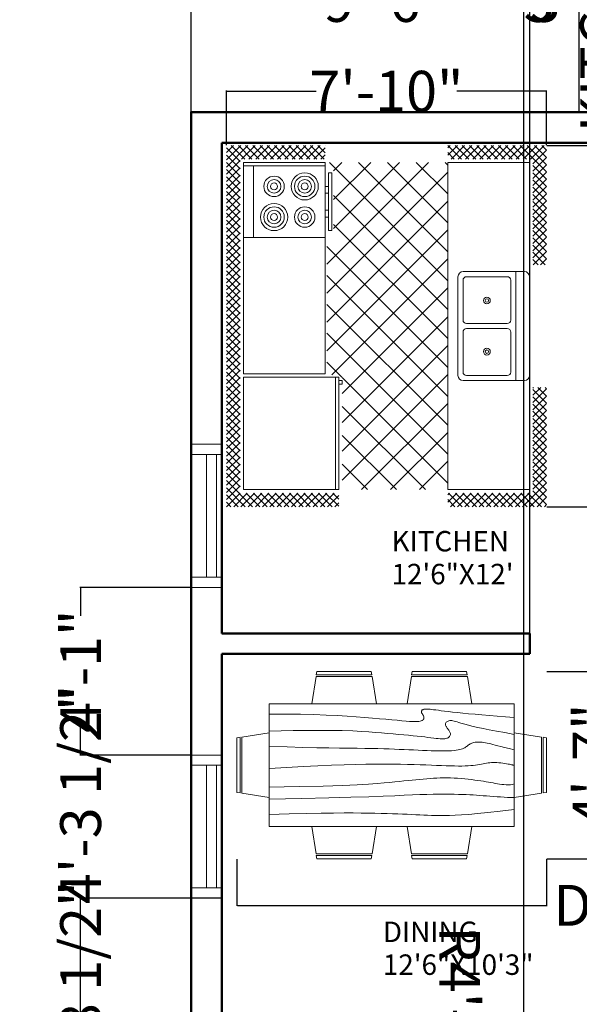
# Model space of a CAD drawing. Units: inches. Extents: x -51 to 1118, y -44 to 791.
# Tile 4 of 8: x -22 to 142, y 344 to 633. Entities that reach past the tile are written whole.
import ezdxf

# ---------------------------------------------------------------- set-up
doc = ezdxf.new("R2010")
doc.units = ezdxf.units.IN
doc.header["$MEASUREMENT"] = 0
for name, color, linetype, lineweight in [('A-ANNO-DIMS', 2, 'Continuous', 18), ('A-AREA-IDEN', 7, 'Continuous', 18), ('A-FLOR-FIXT', 9, 'Continuous', 18), ('A-FURN', 8, 'Continuous', 18), ('A-GLAZ', 4, 'Continuous', 18), ('A-WALL', 7, 'Continuous', 50)]:
    doc.layers.add(name, color=color, linetype=linetype, lineweight=lineweight)
doc.styles.get("Standard").update_dxf_attribs({"font": 'arial.ttf'})
doc.dimstyles.get("Standard").update_dxf_attribs({"dimtxt": 12, "dimasz": 0.18, "dimexe": 0.18, "dimexo": 0.0625, "dimgap": 0.09, "dimtad": 0, "dimdec": 1, "dimzin": 0, "dimdsep": 46, "dimlunit": 3, "dimtxsty": 'Standard', "dimcen": 0.09, "dimadec": 0, "dimazin": 0, "dimtfac": 1, "dimtdec": 1, "dimtofl": 0, "dimtmove": 0, "dimatfit": 3, "dimfxl": 1, "dimtolj": 1, "dimtzin": 0, "dimarcsym": 0})

# ---------------------------------------------------------------- blocks, each defined once
blk = doc.blocks.new('Kitchen Layout - 7 x 8 ft')
for p, q in [((-5, 81.32), (2.68, 89)), ((-5, 83.44), (0.56, 89)), ((-5, 85.56), (-1.56, 89)), ((-5, 87.68), (-3.68, 89)), ((-1, 84.97), (-5, 88.97)), ((-1, 82.85), (-5, 86.85)), ((1.09, 85), (-2.91, 89)), ((3.21, 85), (-0.79, 89)), ((0.81, 85), (4.81, 89)), ((5.34, 85), (1.34, 89)), ((2.93, 85), (6.93, 89)), ((7.46, 85), (3.46, 89)), ((5.05, 85), (9.05, 89)), ((9.58, 85), (5.58, 89)), ((7.17, 85), (11.17, 89)), ((11.7, 85), (7.7, 89)), ((9.29, 85), (13.29, 89)), ((13.82, 85), (9.82, 89)), ((11.41, 85), (15.41, 89)), ((15.94, 85), (11.94, 89)), ((13.53, 85), (17.53, 89)), ((18.06, 85), (14.06, 89)), ((15.65, 85), (19.65, 89)), ((20.18, 85), (16.18, 89)), ((17.78, 85), (21.78, 89)), ((22.31, 85), (18.31, 89)), ((19.9, 85), (23.9, 89)), ((24.43, 85), (20.43, 89)), ((22.02, 85), (26.02, 89)), ((26.55, 85), (22.55, 89)), ((24.14, 85), (28.14, 89)), ((28.67, 85), (24.67, 89)), ((26.26, 85), (30.26, 89)), ((30.79, 85), (26.79, 89)), ((28.38, 85), (32.38, 89)), ((32.91, 85), (28.91, 89)), ((30.5, 85), (34.5, 89)), ((35.03, 85), (31.03, 89)), ((32.63, 85), (36.63, 89)), ((37.16, 85), (33.16, 89)), ((34.75, 85), (38.75, 89)), ((39.28, 85), (35.28, 89)), ((36.87, 85), (40.87, 89)), ((41.4, 85), (37.4, 89)), ((38.99, 85), (42.99, 89)), ((43.52, 85), (39.52, 89)), ((41.11, 85), (45.11, 89)), ((45.64, 85), (41.64, 89)), ((43.23, 85), (47.23, 89)), ((47.76, 85), (43.76, 89)), ((45.35, 85), (49.35, 89)), ((49.88, 85), (45.88, 89)), ((47.47, 85), (51.47, 89)), ((52, 85), (48, 89)), ((49.6, 85), (53.6, 89)), ((54.13, 85), (50.13, 89)), ((51.72, 85), (55.72, 89)), ((56.25, 85), (52.25, 89)), ((53.84, 85), (57.84, 89)), ((58.37, 85), (54.37, 89)), ((55.96, 85), (59.96, 89)), ((60.49, 85), (56.49, 89)), ((58.08, 85), (62.08, 89)), ((62.61, 85), (58.61, 89)), ((60.2, 85), (64.2, 89)), ((64.73, 85), (60.73, 89)), ((62.32, 85), (66.32, 89)), ((66.85, 85), (62.85, 89)), ((64.45, 85), (68.45, 89)), ((68.97, 85), (64.97, 89)), ((66.57, 85), (70.57, 89)), ((71.1, 85), (67.1, 89)), ((68.69, 85), (72.69, 89)), ((73.22, 85), (69.22, 89)), ((70.81, 85), (74.81, 89)), ((75.34, 85), (71.34, 89)), ((72.93, 85), (76.93, 89)), ((77.46, 85), (73.46, 89)), ((75.05, 85), (79.05, 89)), ((79.58, 85), (75.58, 89)), ((77.17, 85), (81.17, 89)), ((81.7, 85), (77.7, 89)), ((79.29, 85), (83.29, 89)), ((83.82, 85), (79.82, 89)), ((81.42, 85), (85.42, 89)), ((85.95, 85), (81.95, 89)), ((83.54, 85), (87.54, 89)), ((88.07, 85), (84.07, 89)), ((85.66, 85), (89.66, 89)), ((90.19, 85), (86.19, 89)), ((87.78, 85), (91.78, 89)), ((92.31, 85), (88.31, 89)), ((89.9, 85), (93.9, 89)), ((94.43, 85), (90.43, 89)), ((92.02, 85), (96.02, 89)), ((96.55, 85), (92.55, 89)), ((94.14, 85), (98.14, 89)), ((101, 82.67), (94.67, 89)), ((96.27, 85), (100.27, 89)), ((101, 84.79), (96.79, 89)), ((97, 83.61), (101, 87.61)), ((101, 86.92), (98.92, 89)), ((-1, 80.73), (-5, 84.73)), ((34, 84), (96, 84)), ((34, 60), (34, 84)), ((96, 84), (96, 60)), ((97, 81.49), (101, 85.49)), ((101, 80.55), (97, 84.55)), ((-5, 79.19), (-1, 83.19)), ((-1, 78.61), (-5, 82.61)), ((-5, 77.07), (-1, 81.07)), ((74, 81), (95, 81)), ((97, 79.37), (101, 83.37)), ((101, 78.43), (97, 82.43)), ((97, 77.25), (101, 81.25)), ((-1, 76.49), (-5, 80.49)), ((-5, 74.95), (-1, 78.95)), ((-1, 74.36), (-5, 78.36)), ((101, 76.31), (97, 80.31)), ((97, 75.13), (101, 79.13)), ((101, 74.19), (97, 78.19)), ((-5, 72.83), (-1, 76.83)), ((-1, 72.24), (-5, 76.24)), ((97, 73.01), (101, 77.01)), ((101, 72.07), (97, 76.07)), ((-5, 70.71), (-1, 74.71)), ((-1, 70.12), (-5, 74.12)), ((-5, 68.59), (-1, 72.59)), ((97, 70.89), (101, 74.89)), ((101, 69.95), (97, 73.95)), ((97, 68.76), (101, 72.76)), ((-1, 68), (-5, 72)), ((-5, 66.47), (-1, 70.47)), ((-1, 65.88), (-5, 69.88)), ((101, 67.82), (97, 71.82)), ((97, 66.64), (101, 70.64)), ((101, 65.7), (97, 69.7)), ((-5, 64.35), (-1, 68.35)), ((-1, 63.76), (-5, 67.76)), ((97, 64.52), (101, 68.52)), ((101, 63.58), (97, 67.58)), ((-5, 62.22), (-1, 66.22)), ((-1, 61.64), (-5, 65.64)), ((-5, 60.1), (-1, 64.1)), ((97, 62.4), (101, 66.4)), ((101, 61.46), (97, 65.46)), ((97, 60.28), (101, 64.28)), ((-1, 59.52), (-5, 63.52)), ((-5, 57.98), (-1, 61.98)), ((-1, 57.39), (-5, 61.39)), ((100.34, 60), (97, 63.34)), ((98.22, 60), (97, 61.22)), ((98.84, 60), (101, 62.16)), ((-1.73, 56), (-5, 59.27)), ((-4.86, 56), (-1, 59.86)), ((10.4, 24), (45.9, 59.5)), ((18.88, 24), (54.38, 59.5)), ((27.37, 24), (62.87, 59.5)), ((33.03, 55.11), (37.41, 59.5)), ((67.71, 24), (33.68, 58.04)), ((96, 60), (34, 60)), ((35.85, 24), (71.35, 59.5)), ((76.2, 24), (40.7, 59.5)), ((84.68, 24), (49.18, 59.5)), ((93.17, 24), (57.67, 59.5)), ((61.31, 24), (96, 58.69)), ((96, 29.65), (66.15, 59.5)), ((80, 60), (80, 59)), ((82, 59), (82, 60)), ((87, 59), (87, 60)), ((89, 60), (89, 59)), ((100.96, 60), (101, 60.04)), ((-3.85, 56), (-5, 57.15)), ((-2.74, 56), (-1, 57.74)), ((0, 57), (33, 57)), ((0, 30.57), (24.43, 55)), ((0, 39.06), (15.94, 55)), ((0, 47.54), (7.46, 55)), ((1.91, 24), (32.91, 55)), ((33.77, 24), (2.77, 55)), ((42.26, 24), (11.26, 55)), ((50.74, 24), (19.74, 55)), ((59.23, 24), (28.23, 55)), ((31, 55), (31, 56)), ((32, 55), (31, 55)), ((32, 56), (32, 55)), ((44.34, 24), (77.84, 57.5)), ((52.82, 24), (86.32, 57.5)), ((96, 38.14), (76.64, 57.5)), ((96, 46.63), (85.13, 57.5)), ((96, 55.11), (93.57, 57.54)), ((25.29, 24), (0, 49.29)), ((69.79, 24), (96, 50.21)), ((16.8, 24), (0, 40.8)), ((78.28, 24), (96, 41.72)), ((8.32, 24), (0, 32.32)), ((86.76, 24), (96, 33.24)), ((-5, 21.92), (-2.92, 24)), ((-5, 19.8), (-1, 23.8)), ((-1, 19.21), (-5, 23.21)), ((-1, 21.33), (-3.67, 24)), ((-1, 23.45), (-1.55, 24)), ((0, 24), (96, 24)), ((0, 0), (0, 24)), ((95.25, 24), (96, 24.75)), ((96, 24), (96, 0)), ((97, 22.1), (98.9, 24)), ((97, 19.97), (101, 23.97)), ((101, 21.16), (98.16, 24)), ((101, 23.28), (100.28, 24)), ((-5, 17.68), (-1, 21.68)), ((-1, 17.09), (-5, 21.09)), ((101, 19.03), (97, 23.03)), ((97, 17.85), (101, 21.85)), ((101, 16.91), (97, 20.91)), ((-5, 15.55), (-1, 19.55)), ((-1, 14.97), (-5, 18.97)), ((-5, 13.43), (-1, 17.43)), ((47.25, 6.5), (47.25, 18.5)), ((48.75, 18.5), (48.75, 6.5)), ((97, 15.73), (101, 19.73)), ((101, 14.79), (97, 18.79)), ((97, 13.61), (101, 17.61)), ((-1, 12.85), (-5, 16.85)), ((-5, 11.31), (-1, 15.31)), ((-1, 10.73), (-5, 14.73)), ((101, 12.67), (97, 16.67)), ((97, 11.49), (101, 15.49)), ((101, 10.55), (97, 14.55)), ((-5, 9.19), (-1, 13.19)), ((-1, 8.6), (-5, 12.6)), ((97, 9.37), (101, 13.37)), ((101, 8.43), (97, 12.43)), ((-5, 7.07), (-1, 11.07)), ((-1, 6.48), (-5, 10.48)), ((-5, 4.95), (-1, 8.95)), ((97, 7.25), (101, 11.25)), ((101, 6.31), (97, 10.31)), ((97, 5.12), (101, 9.12)), ((-1, 4.36), (-5, 8.36)), ((-5, 2.83), (-1, 6.83)), ((-1, 2.24), (-5, 6.24)), ((101, 4.18), (97, 8.18)), ((97, 3), (101, 7)), ((101, 2.06), (97, 6.06)), ((-5, 0.71), (-1, 4.71)), ((-1, 0.12), (-5, 4.12)), ((64, 4), (32, 4)), ((97, 0.88), (101, 4.88)), ((101, -0.06), (97, 3.94)), ((-5, -1.42), (-1, 2.58)), ((2, -5), (-5, 2)), ((-5, -3.54), (-1, 0.46)), ((96, 0), (0, 0)), ((93.24, -5), (101, 2.76)), ((95.36, -5), (101, 0.64)), ((101, -2.18), (97, 1.82)), ((-0.12, -5), (-5, -0.12)), ((-2.25, -5), (-5, -2.25)), ((-4.34, -5), (-0.34, -1)), ((-2.22, -5), (1.78, -1)), ((-0.1, -5), (3.9, -1)), ((4.12, -5), (0.12, -1)), ((2.02, -5), (6.02, -1)), ((6.24, -5), (2.24, -1)), ((4.14, -5), (8.14, -1)), ((8.36, -5), (4.36, -1)), ((6.27, -5), (10.27, -1)), ((10.48, -5), (6.48, -1)), ((8.39, -5), (12.39, -1)), ((12.6, -5), (8.6, -1)), ((10.51, -5), (14.51, -1)), ((14.73, -5), (10.73, -1)), ((12.63, -5), (16.63, -1)), ((16.85, -5), (12.85, -1)), ((14.75, -5), (18.75, -1)), ((18.97, -5), (14.97, -1)), ((16.87, -5), (20.87, -1)), ((21.09, -5), (17.09, -1)), ((18.99, -5), (22.99, -1)), ((23.21, -5), (19.21, -1)), ((21.11, -5), (25.11, -1)), ((25.33, -5), (21.33, -1)), ((23.24, -5), (27.24, -1)), ((27.45, -5), (23.45, -1)), ((25.36, -5), (29.36, -1)), ((29.57, -5), (25.57, -1)), ((27.48, -5), (30, -2.48)), ((30, -3.3), (27.7, -1)), ((30, -1.18), (29.82, -1)), ((66, -2.54), (67.54, -1)), ((66, -4.66), (69.66, -1)), ((69.88, -5), (66, -1.12)), ((67.78, -5), (71.78, -1)), ((72, -5), (68, -1)), ((69.9, -5), (73.9, -1)), ((74.12, -5), (70.12, -1)), ((72.03, -5), (76.03, -1)), ((76.24, -5), (72.24, -1)), ((74.15, -5), (78.15, -1)), ((78.36, -5), (74.36, -1)), ((76.27, -5), (80.27, -1)), ((80.49, -5), (76.49, -1)), ((78.39, -5), (82.39, -1)), ((82.61, -5), (78.61, -1)), ((80.51, -5), (84.51, -1)), ((84.73, -5), (80.73, -1)), ((82.63, -5), (86.63, -1)), ((86.85, -5), (82.85, -1)), ((84.75, -5), (88.75, -1)), ((88.97, -5), (84.97, -1)), ((86.88, -5), (90.88, -1)), ((91.09, -5), (87.09, -1)), ((89, -5), (93, -1)), ((93.21, -5), (89.21, -1)), ((91.12, -5), (95.12, -1)), ((95.34, -5), (91.34, -1)), ((97.46, -5), (93.46, -1)), ((99.58, -5), (95.58, -1)), ((101, -4.3), (97, -0.3)), ((97.48, -5), (101, -1.48)), ((-4.37, -5), (-5, -4.37)), ((29.6, -5), (30, -4.6)), ((67.76, -5), (66, -3.24)), ((99.6, -5), (101, -3.6))]:
    blk.add_line(p, q)
for points in [[(0, 56), (0, 84), (33, 84), (33, 56)], [(74, 60), (74, 84), (95, 84), (95, 60)], [(76, 58), (76, 59), (93, 59), (93, 58)]]:
    blk.add_lwpolyline(points, close=True)
for points in [[(33.5, 21), (62.5, 21)], [(32, 1.5), (32, 19.5)], [(33.5, 6.5), (33.5, 18.5)], [(34.5, 19.5), (46.25, 19.5)], [(49.75, 19.5), (61.5, 19.5)], [(62.5, 18.5), (62.5, 6.5)], [(64, 19.5), (64, 1.5)], [(46.25, 5.5), (34.5, 5.5)], [(61.5, 5.5), (49.75, 5.5)], [(62.5, 0), (33.5, 0)]]:
    blk.add_lwpolyline(points)
for centre, radius in [((80, 75), 4), ((80, 75), 3), ((80, 75), 2), ((80, 75), 1), ((89, 75), 3), ((89, 75), 2), ((89, 75), 1), ((89, 66), 4), ((80, 66), 3), ((80, 66), 2), ((80, 66), 1), ((89, 66), 3), ((89, 66), 2), ((89, 66), 1), ((40.5, 12.5), 1), ((40.5, 12.5), 0.5), ((55.5, 12.5), 1), ((55.5, 12.5), 0.5)]:
    blk.add_circle(centre, radius)
for centre, radius, start, end in [((33.5, 19.5), 1.5, 90, 180), ((62.5, 19.5), 1.5, 0, 90), ((34.5, 18.5), 1, 90, 180), ((46.25, 18.5), 1, 0, 90), ((49.75, 18.5), 1, 90, 180), ((61.5, 18.5), 1, 0, 90), ((34.5, 6.5), 1, 180, 270), ((46.25, 6.5), 1, 270, 0), ((49.75, 6.5), 1, 180, 270), ((61.5, 6.5), 1, 270, 0), ((33.5, 1.5), 1.5, 180, 270), ((62.5, 1.5), 1.5, 270, 0)]:
    blk.add_arc(centre, radius, start, end)
blk = doc.blocks.new('Dining Set - 36 x 72 in.')
for p, q in [((-22, 27.5), (-22.1562, 26.50042)), ((-5.8416, 26.5), (-22.1534, 26.5)), ((-22, 27.5), (-6, 27.5)), ((-5.8437, 26.49966), (-6, 27.5)), ((6, 27.5), (5.8438, 26.50042)), ((22.1584, 26.5), (5.8466, 26.5)), ((6, 27.5), (22, 27.5)), ((22.1563, 26.49966), (22, 27.5)), ((-22.2343, 26.00059), (-23.4847, 17.99762)), ((-22.2304, 26), (-5.7608, 26)), ((-4.5152, 17.99762), (-5.7655, 25.99926)), ((5.7657, 26.00059), (4.5153, 17.99762)), ((5.7696, 26), (22.2392, 26)), ((23.4848, 17.99762), (22.2345, 25.99926)), ((36, 18), (-36, 18)), ((-36, 18), (-36, -18)), ((36, -18), (36, 18)), ((-44.0006, 8.23428), (-35.9976, 9.48474)), ((44.0006, 8.23428), (35.9976, 9.48474)), ((-45.5, 8), (-44.5004, 8.15617)), ((-45.5, 8), (-45.5, -8)), ((-44.5, -8.15843), (-44.5, 8.15338)), ((-44, 8.23041), (-44, -8.23915)), ((44, 8.23041), (44, -8.23915)), ((44.5, -8.15843), (44.5, 8.15338)), ((45.5, 8), (44.5005, 8.15617)), ((45.5, 8), (45.5, -8)), ((-44.4997, -8.15631), (-45.5, -8)), ((-35.9976, -9.48476), (-43.9993, -8.2345)), ((35.9976, -9.48476), (43.9993, -8.2345)), ((44.4997, -8.15631), (45.5, -8)), ((-36, -18), (36, -18)), ((-22.2343, -26.0006), (-23.4847, -17.99762)), ((-4.5152, -17.99762), (-5.7655, -25.99928)), ((5.7657, -26.0006), (4.5153, -17.99762)), ((23.4848, -17.99762), (22.2345, -25.99928)), ((-22.2304, -26), (-5.7608, -26)), ((5.7696, -26), (22.2392, -26)), ((-22, -27.5), (-22.1562, -26.50044)), ((-5.8416, -26.5), (-22.1534, -26.5)), ((-22, -27.5), (-6, -27.5)), ((-5.8437, -26.49967), (-6, -27.5)), ((6, -27.5), (5.8438, -26.50044)), ((22.1584, -26.5), (5.8466, -26.5)), ((6, -27.5), (22, -27.5)), ((22.1563, -26.49967), (22, -27.5))]:
    blk.add_line(p, q)
for points in [[(-36, 15), (-31.1772, 14.97754), (-26.8079, 14.91406), (-22.8538, 14.81543), (-19.276, 14.6875), (-16.0362, 14.53613), (-13.0957, 14.36718), (-10.4159, 14.18652), (-7.9583, 14), (-5.6904, 13.81315), (-3.6035, 13.63021), (-1.6954, 13.45508), (0.0365, 13.29166), (1.5945, 13.14388), (2.9811, 13.01562), (4.1988, 12.9108), (5.25, 12.83333), (6.1393, 12.78613), (6.8802, 12.76823), (7.4883, 12.77767), (7.9792, 12.8125), (8.3685, 12.87077), (8.6719, 12.95052), (8.9049, 13.0498), (9.0833, 13.16666), (9.2205, 13.29899), (9.3216, 13.44401), (9.3895, 13.59879), (9.4271, 13.76041), (9.4373, 13.92594), (9.4232, 14.09245), (9.3875, 14.257), (9.3333, 14.41666), (9.2638, 14.56917), (9.1836, 14.71484), (9.0975, 14.85465), (9.0104, 14.98958), (8.9272, 15.1206), (8.8529, 15.2487), (8.7922, 15.37483), (8.75, 15.5), (8.7305, 15.62467), (8.7344, 15.74739), (8.7617, 15.86621), (8.8125, 15.97916), (8.8867, 16.08431), (8.9844, 16.17968), (9.1055, 16.26334), (9.25, 16.33333), (9.4189, 16.38802), (9.6172, 16.42708), (9.8506, 16.45052), (10.125, 16.45833), (10.4463, 16.45052), (10.8203, 16.42708), (11.2529, 16.38802), (11.75, 16.33333), (12.3184, 16.26318), (12.9694, 16.17838), (13.7151, 16.07991), (14.5677, 15.96875), (15.5395, 15.84586), (16.6426, 15.71224), (17.8893, 15.56884), (19.2917, 15.41666), (20.859, 15.25667), (22.5879, 15.08984), (24.4721, 14.91715), (26.5052, 14.73958), (28.6809, 14.5581), (30.9929, 14.3737), (33.4347, 14.18733), (36, 14)], [(-36, 10), (-28.9766, 10.14274), (-23.1725, 10.20442), (-18.4241, 10.19775), (-14.5677, 10.13541), (-11.4399, 10.03011), (-8.877, 9.89453), (-6.7154, 9.74137), (-4.7917, 9.58333), (-2.9698, 9.43082), (-1.2246, 9.28515), (0.4415, 9.14534), (2.026, 9.01041), (3.5266, 8.87939), (4.9408, 8.7513), (6.266, 8.62516), (7.5, 8.5), (8.6411, 8.37549), (9.6914, 8.2539), (10.6538, 8.13818), (11.5312, 8.03125), (12.3267, 7.93603), (13.043, 7.85547), (13.6831, 7.79248), (14.25, 7.75), (14.7471, 7.7303), (15.1797, 7.73307), (15.5537, 7.75732), (15.875, 7.80208), (16.1494, 7.86637), (16.3828, 7.94922), (16.5811, 8.04964), (16.75, 8.16666), (16.8944, 8.29915), (17.0143, 8.44531), (17.1089, 8.60319), (17.1771, 8.77083), (17.218, 8.94629), (17.2305, 9.1276), (17.2137, 9.31282), (17.1667, 9.5), (17.0895, 9.6875), (16.987, 9.875), (16.8649, 10.0625), (16.7292, 10.25), (16.5856, 10.4375), (16.4401, 10.625), (16.2985, 10.8125), (16.1667, 11), (16.05, 11.18733), (15.9518, 11.3737), (15.8752, 11.5581), (15.8229, 11.73958), (15.798, 11.91715), (15.8034, 12.08984), (15.842, 12.25667), (15.9167, 12.41666), (16.0295, 12.56836), (16.1784, 12.70833), (16.3605, 12.83268), (16.5729, 12.9375), (16.8127, 13.01888), (17.0768, 13.07291), (17.3625, 13.0957), (17.6667, 13.08333), (17.9894, 13.03312), (18.3418, 12.94726), (18.7382, 12.82918), (19.1927, 12.68229), (19.7195, 12.51001), (20.3327, 12.31575), (21.0465, 12.10294), (21.875, 11.875), (22.8357, 11.63354), (23.959, 11.37304), (25.2786, 11.08618), (26.8282, 10.76562), (28.6414, 10.40405), (30.752, 9.99414), (33.1936, 9.52856), (36, 9)], [(-36, 5.5), (-30.7157, 5.3348), (-26.069, 5.20963), (-21.9946, 5.11767), (-18.4271, 5.05208), (-15.3009, 5.00602), (-12.5508, 4.97265), (-10.1112, 4.94515), (-7.9167, 4.91666), (-5.909, 4.88167), (-4.0586, 4.83984), (-2.3429, 4.79215), (-0.7396, 4.73958), (0.7739, 4.6831), (2.22, 4.6237), (3.6213, 4.56233), (5, 4.5), (6.373, 4.43782), (7.7344, 4.3776), (9.0723, 4.32129), (10.375, 4.27083), (11.6309, 4.22819), (12.8281, 4.19531), (13.9551, 4.17415), (15, 4.16666), (15.954, 4.17448), (16.819, 4.19791), (17.6001, 4.23698), (18.3021, 4.29166), (18.9299, 4.36198), (19.4883, 4.44791), (19.9823, 4.54948), (20.4167, 4.66666), (20.7969, 4.79899), (21.1302, 4.94401), (21.4245, 5.09879), (21.6875, 5.26041), (21.9271, 5.42594), (22.1511, 5.59245), (22.3672, 5.757), (22.5834, 5.91666), (22.8065, 6.06868), (23.0404, 6.21093), (23.2879, 6.34147), (23.5521, 6.45833), (23.8358, 6.55957), (24.142, 6.64323), (24.4735, 6.70735), (24.8334, 6.75), (25.2235, 6.76969), (25.642, 6.76692), (26.0858, 6.74267), (26.5521, 6.69791), (27.0379, 6.63362), (27.5404, 6.55078), (28.0565, 6.45036), (28.5834, 6.33333), (29.1242, 6.19987), (29.7071, 6.04687), (30.3661, 5.87044), (31.1354, 5.66666), (32.0493, 5.43164), (33.142, 5.16146), (34.4475, 4.85221), (36, 4.5)], [(-36, -1), (-30.7915, -0.6591), (-26.0195, -0.38216), (-21.6519, -0.16284), (-17.6563, 0.00521), (-14.0005, 0.12833), (-10.6523, 0.21289), (-7.5796, 0.26522), (-4.75, 0.29166), (-2.134, 0.29793), (0.2878, 0.28711), (2.5317, 0.26163), (4.6146, 0.22396), (6.5529, 0.17651), (8.3633, 0.12174), (10.0623, 0.06209), (11.6667, 0), (13.1899, -0.06201), (14.6341, -0.1211), (15.9982, -0.17432), (17.2813, -0.21875), (18.4823, -0.25147), (19.6003, -0.26953), (20.6343, -0.27002), (21.5834, -0.25), (22.4481, -0.20768), (23.2357, -0.14584), (23.9549, -0.06836), (24.6146, 0.02083), (25.2235, 0.11784), (25.7904, 0.21875), (26.3241, 0.31966), (26.8334, 0.41666), (27.3265, 0.50618), (27.8099, 0.58593), (28.2894, 0.65397), (28.7709, 0.70833), (29.2601, 0.74707), (29.763, 0.76823), (30.2855, 0.76985), (30.8334, 0.75), (31.4088, 0.70784), (31.9994, 0.64713), (32.589, 0.57275), (33.1615, 0.48958), (33.7008, 0.4025), (34.1908, 0.3164), (34.6153, 0.23616), (34.9584, 0.16666), (35.2099, 0.11165), (35.3848, 0.07031), (35.504, 0.04069), (35.5886, 0.02083), (35.6594, 0.00879), (35.7377, 0.0026), (35.8442, 0.00032), (36, 0)], [(-36, -6.5), (-27.1843, -6.31267), (-20.084, -6.1263), (-14.469, -5.9419), (-10.1094, -5.76042), (-6.7752, -5.58285), (-4.2363, -5.41016), (-2.2629, -5.24333), (-0.625, -5.08334), (0.8708, -4.93099), (2.2715, -4.78646), (3.5872, -4.64974), (4.8281, -4.52084), (6.0046, -4.39974), (7.127, -4.28646), (8.2053, -4.18099), (9.25, -4.08334), (10.2705, -3.99382), (11.2734, -3.91407), (12.2647, -3.84603), (13.25, -3.79167), (14.2354, -3.75293), (15.2266, -3.73177), (16.2295, -3.73015), (17.25, -3.75), (18.2912, -3.79248), (19.3451, -3.85547), (20.4009, -3.93604), (21.4479, -4.03125), (22.4754, -4.13819), (23.4727, -4.25391), (24.4289, -4.37549), (25.3334, -4.5), (26.1785, -4.62492), (26.9694, -4.74935), (27.7145, -4.87281), (28.4219, -4.99479), (29.1, -5.11483), (29.7572, -5.23242), (30.4016, -5.34709), (31.0417, -5.45834), (31.6837, -5.56437), (32.3262, -5.65821), (32.9658, -5.73153), (33.599, -5.77604), (34.2224, -5.78345), (34.8327, -5.74545), (35.4264, -5.65373), (36, -5.5)], [(-36, -10), (-26.4022, -9.81299), (-18.4675, -9.62891), (-11.9839, -9.45069), (-6.7396, -9.28125), (-2.5226, -9.12354), (0.8789, -8.98047), (3.6769, -8.85498), (6.0833, -8.75), (8.2767, -8.66765), (10.3021, -8.60677), (12.1712, -8.56543), (13.8958, -8.54167), (15.4876, -8.53353), (16.9583, -8.53907), (18.3197, -8.55632), (19.5834, -8.58334), (20.7616, -8.61841), (21.8685, -8.66081), (22.9188, -8.71004), (23.9271, -8.76563), (24.9081, -8.82707), (25.8763, -8.89388), (26.8465, -8.96558), (27.8334, -9.04167), (28.8474, -9.12118), (29.8828, -9.20117), (30.93, -9.27824), (31.9792, -9.34896), (33.0205, -9.40991), (34.0443, -9.45768), (35.0407, -9.48885), (36, -9.5)], [(-36, -14.5), (-30.0881, -14.33513), (-25.0332, -14.21224), (-20.7312, -14.12647), (-17.0781, -14.07292), (-13.97, -14.04671), (-11.3027, -14.04297), (-8.9724, -14.05681), (-6.875, -14.08334), (-4.9224, -14.11833), (-3.0905, -14.16016), (-1.3709, -14.20785), (0.2448, -14.26042), (1.7647, -14.3169), (3.1973, -14.3763), (4.5507, -14.43767), (5.8333, -14.5), (7.0554, -14.5621), (8.235, -14.62175), (9.3922, -14.67652), (10.5469, -14.72396), (11.7192, -14.76164), (12.929, -14.78711), (14.1965, -14.79794), (15.5417, -14.79167), (16.9933, -14.76424), (18.6152, -14.70508), (20.4804, -14.60197), (22.6615, -14.44271), (25.2312, -14.21509), (28.2624, -13.9069), (31.8277, -13.50594), (36, -13)]]:
    blk.add_lwpolyline(points)
blk = doc.blocks.new('*D10')
at = {"layer": 'A-ANNO-DIMS', "color": 0, "lineweight": -2, "transparency": 16777216}
for p, q in [((28.02, 606), (28.02, 654.38)), ((28.2, 654.2), (173.65, 654.2)), ((339.84, 654.2), (194.4, 654.2)), ((340.02, 606), (340.02, 654.38))]:
    blk.add_line(p, q, dxfattribs=at)
at = {"layer": 'A-ANNO-DIMS', "color": 0, "transparency": 16777216}
for points in [[(28.2, 654.23), (28.2, 654.17), (28.02, 654.2)], [(339.84, 654.23), (339.84, 654.17), (340.02, 654.2)]]:
    blk.add_solid(points, dxfattribs=at)
at = {"layer": 'Defpoints', "color": 0, "transparency": 16777216}
for p in [(340.02, 654.2), (28.02, 605.94), (340.02, 605.94)]:
    blk.add_point(p, dxfattribs=at)
at = {"layer": 'A-ANNO-DIMS', "color": 0, "transparency": 16777216, "insert": (184.02, 654.2), "char_height": 12, "attachment_point": 5}
blk.add_mtext("\\A1;26'", dxfattribs=at)
blk = doc.blocks.new('WIN-36IN')
for p, q in [((9, 42), (0, 42)), ((9, 39), (0, 39)), ((0, 39), (0, 3)), ((4.5, 3), (4.5, 39)), ((7.5, 3), (7.5, 39)), ((9, 3), (9, 39)), ((0, 3), (9, 3)), ((0, 0), (9, 0))]:
    blk.add_line(p, q)
blk = doc.blocks.new('*D34')
at = {"layer": 'A-ANNO-DIMS', "color": 0, "lineweight": -2, "transparency": 16777216}
for p, q in [((132.45, 596.14), (148.46, 596.14)), ((148.28, 596.14), (148.28, 596.32)), ((148.28, 490.32), (148.28, 595.96)), ((132.45, 490.14), (148.46, 490.14))]:
    blk.add_line(p, q, dxfattribs=at)
at = {"layer": 'A-ANNO-DIMS', "color": 0, "transparency": 16777216}
for points in [[(148.25, 595.96), (148.31, 595.96), (148.28, 596.14)], [(148.25, 490.32), (148.31, 490.32), (148.28, 490.14)]]:
    blk.add_solid(points, dxfattribs=at)
at = {"layer": 'Defpoints', "color": 0, "transparency": 16777216}
for p in [(132.38, 596.14), (148.28, 596.14), (132.38, 490.14)]:
    blk.add_point(p, dxfattribs=at)
at = {"layer": 'A-ANNO-DIMS', "color": 0, "transparency": 16777216, "insert": (148.28, 696.39), "char_height": 12, "attachment_point": 5, "rotation": 90}
blk.add_mtext('\\A1;KITCHEN FITTINGS 8\'-10"', dxfattribs=at)
blk = doc.blocks.new('*D35')
at = {"layer": 'A-ANNO-DIMS', "color": 0, "lineweight": -2, "transparency": 16777216}
for p, q in [((38.38, 596.21), (38.38, 612.22)), ((38.56, 612.04), (64.73, 612.04)), ((132.2, 612.04), (106.04, 612.04)), ((132.38, 596.21), (132.38, 612.22))]:
    blk.add_line(p, q, dxfattribs=at)
at = {"layer": 'A-ANNO-DIMS', "color": 0, "transparency": 16777216}
for points in [[(38.56, 612.07), (38.56, 612.01), (38.38, 612.04)], [(132.2, 612.07), (132.2, 612.01), (132.38, 612.04)]]:
    blk.add_solid(points, dxfattribs=at)
at = {"layer": 'Defpoints', "color": 0, "transparency": 16777216}
for p in [(38.38, 612.04), (38.38, 596.14), (132.38, 596.14)]:
    blk.add_point(p, dxfattribs=at)
at = {"layer": 'A-ANNO-DIMS', "color": 0, "transparency": 16777216, "insert": (85.38, 612.04), "char_height": 12, "attachment_point": 5}
blk.add_mtext('\\A1;7\'-10"', dxfattribs=at)
blk = doc.blocks.new('*D40')
at = {"layer": 'A-ANNO-DIMS', "color": 0, "lineweight": -2, "transparency": 16777216}
for p, q in [((41.43, 386.75), (41.43, 372.98)), ((132.43, 386.75), (132.43, 372.98)), ((41.61, 373.16), (132.25, 373.16)), ((132.43, 373.16), (132.61, 373.16))]:
    blk.add_line(p, q, dxfattribs=at)
at = {"layer": 'A-ANNO-DIMS', "color": 0, "transparency": 16777216}
for points in [[(41.61, 373.19), (41.61, 373.13), (41.43, 373.16)], [(132.25, 373.19), (132.25, 373.13), (132.43, 373.16)]]:
    blk.add_solid(points, dxfattribs=at)
at = {"layer": 'Defpoints', "color": 0, "transparency": 16777216}
for p in [(41.43, 386.81), (132.43, 386.81), (132.43, 373.16)]:
    blk.add_point(p, dxfattribs=at)
at = {"layer": 'A-ANNO-DIMS', "color": 0, "transparency": 16777216, "insert": (198.65, 373.16), "char_height": 12, "attachment_point": 5}
blk.add_mtext('\\A1;DINING SET 7\'-7"', dxfattribs=at)
blk = doc.blocks.new('*D41')
at = {"layer": 'A-ANNO-DIMS', "color": 0, "lineweight": -2, "transparency": 16777216}
for p, q in [((132.49, 441.81), (146.26, 441.81)), ((146.08, 441.63), (146.08, 430.59)), ((146.08, 386.99), (146.08, 398.03)), ((132.49, 386.81), (146.26, 386.81))]:
    blk.add_line(p, q, dxfattribs=at)
at = {"layer": 'A-ANNO-DIMS', "color": 0, "transparency": 16777216}
for points in [[(146.05, 441.63), (146.11, 441.63), (146.08, 441.81)], [(146.05, 386.99), (146.11, 386.99), (146.08, 386.81)]]:
    blk.add_solid(points, dxfattribs=at)
at = {"layer": 'Defpoints', "color": 0, "transparency": 16777216}
for p in [(132.43, 441.81), (146.08, 441.81), (132.43, 386.81)]:
    blk.add_point(p, dxfattribs=at)
at = {"layer": 'A-ANNO-DIMS', "color": 0, "transparency": 16777216, "insert": (146.08, 414.31), "char_height": 12, "attachment_point": 5, "rotation": 90}
blk.add_mtext('\\A1;4\'-7"', dxfattribs=at)
blk = doc.blocks.new('*D45')
at = {"layer": 'A-ANNO-DIMS', "color": 0, "lineweight": -2, "transparency": 16777216}
for p, q in [((36.96, 317.94), (-4.61, 317.94)), ((-4.43, 317.94), (-4.43, 318.12)), ((-4.43, 285.72), (-4.43, 317.76)), ((36.96, 285.54), (-4.61, 285.54))]:
    blk.add_line(p, q, dxfattribs=at)
at = {"layer": 'A-ANNO-DIMS', "color": 0, "transparency": 16777216}
for points in [[(-4.46, 317.76), (-4.4, 317.76), (-4.43, 317.94)], [(-4.46, 285.72), (-4.4, 285.72), (-4.43, 285.54)]]:
    blk.add_solid(points, dxfattribs=at)
at = {"layer": 'Defpoints', "color": 0, "transparency": 16777216}
for p in [(-4.43, 317.94), (37.02, 317.94), (37.02, 285.54)]:
    blk.add_point(p, dxfattribs=at)
at = {"layer": 'A-ANNO-DIMS', "color": 0, "transparency": 16777216, "insert": (-4.43, 348.24), "char_height": 12, "attachment_point": 5, "rotation": 90}
blk.add_mtext('\\A1;2\'-8 1/2"', dxfattribs=at)
blk = doc.blocks.new('*D46')
at = {"layer": 'A-ANNO-DIMS', "color": 0, "lineweight": -2, "transparency": 16777216}
for p, q in [((36.96, 375.28), (-4.61, 375.28)), ((-4.43, 375.28), (-4.43, 375.46)), ((-4.43, 324.12), (-4.43, 375.1)), ((36.96, 323.94), (-4.61, 323.94))]:
    blk.add_line(p, q, dxfattribs=at)
at = {"layer": 'A-ANNO-DIMS', "color": 0, "transparency": 16777216}
for points in [[(-4.46, 375.1), (-4.4, 375.1), (-4.43, 375.28)], [(-4.46, 324.12), (-4.4, 324.12), (-4.43, 323.94)]]:
    blk.add_solid(points, dxfattribs=at)
at = {"layer": 'Defpoints', "color": 0, "transparency": 16777216}
for p in [(-4.43, 375.28), (37.02, 375.28), (37.02, 323.94)]:
    blk.add_point(p, dxfattribs=at)
at = {"layer": 'A-ANNO-DIMS', "color": 0, "transparency": 16777216, "insert": (-4.43, 405.72), "char_height": 12, "attachment_point": 5, "rotation": 90}
blk.add_mtext('\\A1;4\'-3 1/2"', dxfattribs=at)
blk = doc.blocks.new('*D47')
at = {"layer": 'A-ANNO-DIMS', "color": 0, "lineweight": -2, "transparency": 16777216}
for p, q in [((27.96, 466.47), (-4.61, 466.47)), ((-4.43, 466.29), (-4.43, 458.16)), ((-4.43, 417.46), (-4.43, 425.6)), ((27.96, 417.28), (-4.61, 417.28))]:
    blk.add_line(p, q, dxfattribs=at)
at = {"layer": 'A-ANNO-DIMS', "color": 0, "transparency": 16777216}
for points in [[(-4.46, 466.29), (-4.4, 466.29), (-4.43, 466.47)], [(-4.46, 417.46), (-4.4, 417.46), (-4.43, 417.28)]]:
    blk.add_solid(points, dxfattribs=at)
at = {"layer": 'Defpoints', "color": 0, "transparency": 16777216}
for p in [(-4.43, 466.47), (28.02, 466.47), (28.02, 417.28)]:
    blk.add_point(p, dxfattribs=at)
at = {"layer": 'A-ANNO-DIMS', "color": 0, "transparency": 16777216, "insert": (-4.43, 441.88), "char_height": 12, "attachment_point": 5, "rotation": 90}
blk.add_mtext('\\A1;4\'-1"', dxfattribs=at)
blk = doc.blocks.new('*D48')
at = {"layer": 'A-ANNO-DIMS', "color": 0, "lineweight": -2, "transparency": 16777216}
for p, q in [((28.02, 606), (28.02, 638.57)), ((142.02, 606), (142.02, 638.57)), ((28.2, 638.39), (68.98, 638.39)), ((141.84, 638.39), (101.06, 638.39))]:
    blk.add_line(p, q, dxfattribs=at)
at = {"layer": 'A-ANNO-DIMS', "color": 0, "transparency": 16777216}
for points in [[(28.2, 638.42), (28.2, 638.36), (28.02, 638.39)], [(141.84, 638.42), (141.84, 638.36), (142.02, 638.39)]]:
    blk.add_solid(points, dxfattribs=at)
at = {"layer": 'Defpoints', "color": 0, "transparency": 16777216}
for p in [(142.02, 638.39), (28.02, 605.94), (142.02, 605.94)]:
    blk.add_point(p, dxfattribs=at)
at = {"layer": 'A-ANNO-DIMS', "color": 0, "transparency": 16777216, "insert": (85.02, 638.39), "char_height": 12, "attachment_point": 5}
blk.add_mtext('\\A1;9\'-6"', dxfattribs=at)
blk = doc.blocks.new('*D61')
at = {"layer": 'A-ANNO-DIMS', "color": 0, "lineweight": -2, "transparency": 16777216}
for p, q in [((125.75, 324), (125.75, 638.57)), ((161.75, 324), (161.75, 638.57)), ((125.93, 638.39), (127.71, 638.39)), ((161.57, 638.39), (159.79, 638.39))]:
    blk.add_line(p, q, dxfattribs=at)
at = {"layer": 'A-ANNO-DIMS', "color": 0, "transparency": 16777216}
for points in [[(125.93, 638.42), (125.93, 638.36), (125.75, 638.39)], [(161.57, 638.42), (161.57, 638.36), (161.75, 638.39)]]:
    blk.add_solid(points, dxfattribs=at)
at = {"layer": 'Defpoints', "color": 0, "transparency": 16777216}
for p in [(161.75, 638.39), (125.75, 323.94), (161.75, 323.94)]:
    blk.add_point(p, dxfattribs=at)
at = {"layer": 'A-ANNO-DIMS', "color": 0, "transparency": 16777216, "insert": (143.75, 638.39), "char_height": 12, "attachment_point": 5}
blk.add_mtext('\\A1;3\'-0"', dxfattribs=at)
blk = doc.blocks.new('*D63')
at = {"layer": 'A-ANNO-DIMS', "color": 0, "lineweight": -2, "transparency": 16777216}
for p, q in [((127.45, 453), (127.45, 638.57)), ((163.45, 453), (163.45, 638.57)), ((127.63, 638.39), (129.41, 638.39)), ((163.27, 638.39), (161.48, 638.39))]:
    blk.add_line(p, q, dxfattribs=at)
at = {"layer": 'A-ANNO-DIMS', "color": 0, "transparency": 16777216}
for points in [[(127.63, 638.42), (127.63, 638.36), (127.45, 638.39)], [(163.27, 638.42), (163.27, 638.36), (163.45, 638.39)]]:
    blk.add_solid(points, dxfattribs=at)
at = {"layer": 'Defpoints', "color": 0, "transparency": 16777216}
for p in [(163.45, 638.39), (127.45, 452.94), (163.45, 452.94)]:
    blk.add_point(p, dxfattribs=at)
at = {"layer": 'A-ANNO-DIMS', "color": 0, "transparency": 16777216, "insert": (145.45, 638.39), "char_height": 12, "attachment_point": 5}
blk.add_mtext('\\A1;3\'-0"', dxfattribs=at)
blk = doc.blocks.new('*D70')
at = {"layer": 'A-ANNO-DIMS', "color": 0, "lineweight": -2, "transparency": 16777216}
for p, q in [((106.9, 293.87), (106.9, 293.69)), ((106.81, 239.07), (106.99, 239.07)), ((106.9, 238.98), (106.9, 239.16))]:
    blk.add_line(p, q, dxfattribs=at)
at = {"layer": 'A-ANNO-DIMS', "color": 0, "transparency": 16777216}
blk.add_solid([(106.93, 293.69), (106.87, 293.69), (106.9, 293.51)], dxfattribs=at)
at = {"layer": 'Defpoints', "color": 0, "transparency": 16777216}
for p in [(106.9, 293.51), (106.9, 239.07)]:
    blk.add_point(p, dxfattribs=at)
at = {"layer": 'A-ANNO-DIMS', "color": 0, "transparency": 16777216, "insert": (106.9, 329.63), "char_height": 12, "attachment_point": 5, "rotation": 270.0002}
blk.add_mtext('\\A1;R4\'-6 1/2"', dxfattribs=at)

msp = doc.modelspace()

# ---------------------------------------------------------------- linework, layer by layer
at = {"layer": 'A-WALL'}
for p, q in [((37.02, 596.94), (37.02, 452.94)), ((145.02, 596.94), (37.02, 596.94)), ((127.45, 452.94), (37.02, 452.94)), ((127.45, 446.94), (127.45, 452.94)), ((37.02, 446.94), (37.02, 107.94)), ((127.45, 446.94), (37.02, 446.94))]:
    msp.add_line(p, q, dxfattribs=at)
msp.add_lwpolyline([(145.02, 605.94), (28.02, 605.94), (28.02, 5.94), (340.02, 5.94), (340.02, 605.94), (181.02, 605.94)], dxfattribs=at)

# ---------------------------------------------------------------- block references
at = {"layer": 'A-FLOR-FIXT', "rotation": 90}
msp.add_blockref('Kitchen Layout - 7 x 8 ft', (127.38, 495.14), dxfattribs=at)
at = {"layer": 'A-FURN'}
msp.add_blockref('Dining Set - 36 x 72 in.', (86.93, 414.31), dxfattribs=at)
at = {"layer": 'A-GLAZ'}
for p in [(28.02, 466.47), (28.02, 375.28)]:
    msp.add_blockref('WIN-36IN', p, dxfattribs=at)

# ---------------------------------------------------------------- texts
at = {"layer": 'A-AREA-IDEN'}
for s, p in [('KITCHEN', (86.87, 477.01)), ('12\'6"X12\'', (86.87, 467.37)), ('DINING', (84.32, 362.39)), ('12\'6"X10\'3"', (84.32, 352.76))]:
    msp.add_text(s, height=6, dxfattribs=at).set_placement(p)

# ---------------------------------------------------------------- dimensions: what is measured, and where the dimension line sits
at = {"layer": 'A-ANNO-DIMS'}
dim = msp.add_linear_dim(base=(148.28, 596.14), p1=(132.38, 490.14), p2=(132.38, 596.14), angle=90, text='KITCHEN FITTINGS <>', dimstyle='Standard', override={"dimdec": 1, "dimlfac": 1, "dimrnd": 0, "dimzin": 1, "dimdsep": 46, "dimlunit": 4, "dimfrac": 2}, dxfattribs=at)
dim.commit()
dim.dimension.update_dxf_attribs({"geometry": '*D34', "text_midpoint": (148.28, 696.39)})
for base, p1, p2, override, picture, middle in [((340.02, 654.2), (28.02, 605.94), (340.02, 605.94), {"dimclrd": 0, "dimclre": 0, "dimclrt": 0}, '*D10', (184.02, 654.2)), ((142.02, 638.39), (28.02, 605.94), (142.02, 605.94), {"dimdec": 1, "dimlfac": 1, "dimrnd": 0, "dimzin": 1, "dimdsep": 46, "dimlunit": 4, "dimfrac": 2}, '*D48', (85.02, 638.39)), ((161.75, 638.39), (125.75, 323.94), (161.75, 323.94), {"dimdec": 1, "dimlfac": 1, "dimrnd": 0, "dimzin": 1, "dimdsep": 46, "dimlunit": 4, "dimfrac": 2}, '*D61', (143.75, 638.39)), ((163.45, 638.39), (127.45, 452.94), (163.45, 452.94), {"dimdec": 1, "dimlfac": 1, "dimrnd": 0, "dimzin": 1, "dimdsep": 46, "dimlunit": 4, "dimfrac": 2}, '*D63', (145.45, 638.39))]:
    dim = msp.add_linear_dim(base=base, p1=p1, p2=p2, dimstyle='Standard', override=override, dxfattribs=at)
    dim.commit()
    dim.dimension.update_dxf_attribs({"geometry": picture, "text_midpoint": middle})
for base, p1, p2, angle, picture, middle in [((38.38, 612.04), (132.38, 596.14), (38.38, 596.14), 180, '*D35', (85.38, 612.04)), ((-4.43, 466.47), (28.02, 417.28), (28.02, 466.47), 90, '*D47', (-4.43, 441.88)), ((146.08, 441.81), (132.43, 386.81), (132.43, 441.81), 90, '*D41', (146.08, 414.31)), ((-4.43, 375.28), (37.02, 323.94), (37.02, 375.28), 90, '*D46', (-4.43, 405.72)), ((-4.43, 317.94), (37.02, 285.54), (37.02, 317.94), 90, '*D45', (-4.43, 348.24))]:
    dim = msp.add_linear_dim(base=base, p1=p1, p2=p2, angle=angle, dimstyle='Standard', override={"dimdec": 1, "dimlfac": 1, "dimrnd": 0, "dimzin": 1, "dimdsep": 46, "dimlunit": 4, "dimfrac": 2}, dxfattribs=at)
    dim.commit()
    dim.dimension.update_dxf_attribs({"geometry": picture, "text_midpoint": middle})
dim = msp.add_linear_dim(base=(132.43, 373.16), p1=(41.43, 386.81), p2=(132.43, 386.81), text='DINING SET <>', dimstyle='Standard', override={"dimdec": 1, "dimlfac": 1, "dimrnd": 0, "dimzin": 1, "dimdsep": 46, "dimlunit": 4, "dimfrac": 2}, dxfattribs=at)
dim.commit()
dim.dimension.update_dxf_attribs({"geometry": '*D40', "text_midpoint": (198.65, 373.16)})
dim = msp.add_radius_dim(center=(106.9, 239.07), mpoint=(106.9, 293.51), dimstyle='Standard', override={"dimdec": 1, "dimlfac": 1, "dimrnd": 0, "dimzin": 1, "dimdsep": 46, "dimlunit": 4, "dimfrac": 2}, dxfattribs=at)
dim.commit()
dim.dimension.update_dxf_attribs({"geometry": '*D70', "text_midpoint": (106.9, 329.63)})

doc.saveas('drawing.dxf')
